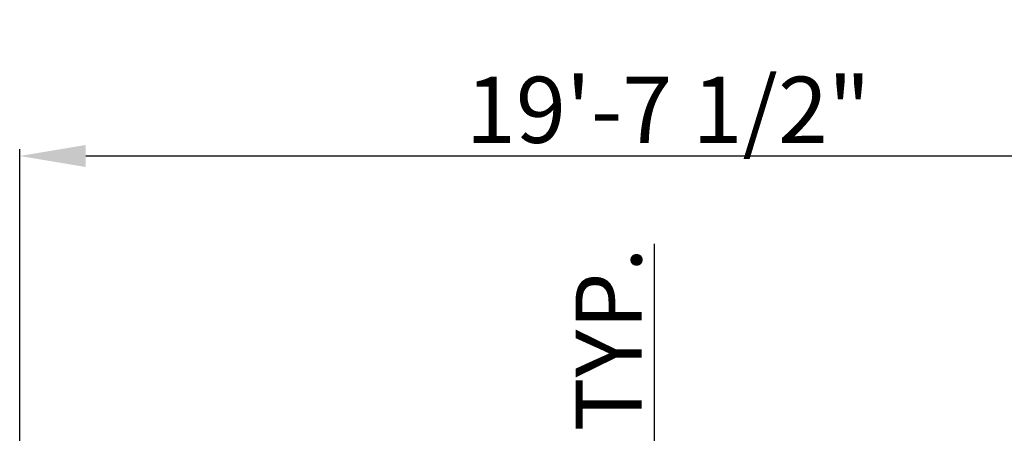
# Model space of a CAD drawing. Units: inches. Extents: x 2083 to 3317, y 1141 to 2115.
# Tile 101 of 256: x 2236 to 2415, y 2023 to 2098. Entities that reach past the tile are written whole.
import ezdxf

# ---------------------------------------------------------------- set-up
doc = ezdxf.new("R2010")
doc.units = ezdxf.units.IN
doc.layers.add('A-ANNO-DIMS', color=2, linetype='Continuous', lineweight=18)
doc.styles.get("Standard").update_dxf_attribs({"font": 'arial.ttf'})
doc.dimstyles.new('ISO-25', dxfattribs={"dimtxt": 12, "dimasz": 12, "dimexe": 1.25, "dimexo": 0.625, "dimtad": 1, "dimlunit": 3, "dimtxsty": 'Standard', "dimcen": 2.5, "dimadec": 0, "dimazin": 0, "dimtfac": 1, "dimtmove": 0, "dimatfit": 3, "dimfxl": 1, "dimarcsym": 0})

# ---------------------------------------------------------------- blocks, each defined once
blk = doc.blocks.new('*D21')
at = {"layer": 'A-ANNO-DIMS', "color": 0, "lineweight": -2, "transparency": 16777216}
for p, q in [((2351.18, 1970.69), (2351.18, 2057.15)), ((2337.85, 1970.69), (2352.43, 1970.69)), ((2351.18, 1909.74), (2351.18, 1958.69)), ((2337.85, 1897.74), (2352.43, 1897.74))]:
    blk.add_line(p, q, dxfattribs=at)
at = {"layer": 'A-ANNO-DIMS', "color": 0, "transparency": 16777216}
for points in [[(2349.18, 1958.69), (2353.18, 1958.69), (2351.18, 1970.69)], [(2349.18, 1909.74), (2353.18, 1909.74), (2351.18, 1897.74)]]:
    blk.add_solid(points, dxfattribs=at)
at = {"layer": 'Defpoints', "color": 0, "transparency": 16777216}
for p in [(2337.22, 1970.69), (2351.18, 1970.69), (2337.22, 1897.74)]:
    blk.add_point(p, dxfattribs=at)
at = {"layer": 'A-ANNO-DIMS', "color": 0, "transparency": 16777216, "insert": (2344.43, 2019.92), "char_height": 12, "attachment_point": 5, "rotation": 90}
blk.add_mtext('6\'-1" TYP.', dxfattribs=at)
blk = doc.blocks.new('*D36')
at = {"layer": 'A-ANNO-DIMS', "color": 0, "lineweight": -2, "transparency": 16777216}
for p, q in [((2235.96, 2012.39), (2235.96, 2074.36)), ((2471.46, 2012.39), (2471.46, 2074.36)), ((2247.96, 2073.11), (2459.46, 2073.11))]:
    blk.add_line(p, q, dxfattribs=at)
at = {"layer": 'A-ANNO-DIMS', "color": 0, "transparency": 16777216}
for points in [[(2247.96, 2075.11), (2247.96, 2071.11), (2235.96, 2073.11)], [(2459.46, 2075.11), (2459.46, 2071.11), (2471.46, 2073.11)]]:
    blk.add_solid(points, dxfattribs=at)
at = {"layer": 'Defpoints', "color": 0, "transparency": 16777216}
for p in [(2471.46, 2073.11), (2235.96, 2011.76), (2471.46, 2011.76)]:
    blk.add_point(p, dxfattribs=at)
at = {"layer": 'A-ANNO-DIMS', "color": 0, "transparency": 16777216, "insert": (2353.71, 2079.94), "char_height": 12, "attachment_point": 5}
blk.add_mtext('19\'-7 1/2"', dxfattribs=at)

msp = doc.modelspace()

# ---------------------------------------------------------------- dimensions: what is measured, and where the dimension line sits
at = {"layer": 'A-ANNO-DIMS'}
dim = msp.add_linear_dim(base=(2471.46, 2073.111), p1=(2235.96, 2011.761), p2=(2471.46, 2011.761), dimstyle='ISO-25', override={"dimdec": 1, "dimlfac": 1, "dimrnd": 0, "dimzin": 1, "dimdsep": 46, "dimlunit": 4, "dimfrac": 2}, dxfattribs=at)
dim.commit()
dim.dimension.update_dxf_attribs({"geometry": '*D36', "text_midpoint": (2353.71, 2079.941)})
dim = msp.add_linear_dim(base=(2351.181, 1970.691), p1=(2337.22, 1897.744), p2=(2337.22, 1970.691), angle=90, text='<> TYP.', dimstyle='ISO-25', override={"dimdec": 1, "dimlfac": 1, "dimrnd": 0, "dimzin": 1, "dimdsep": 46, "dimlunit": 4, "dimfrac": 2}, dxfattribs=at)
dim.commit()
dim.dimension.update_dxf_attribs({"geometry": '*D21', "text_midpoint": (2344.429, 2019.922)})

doc.saveas('drawing.dxf')
